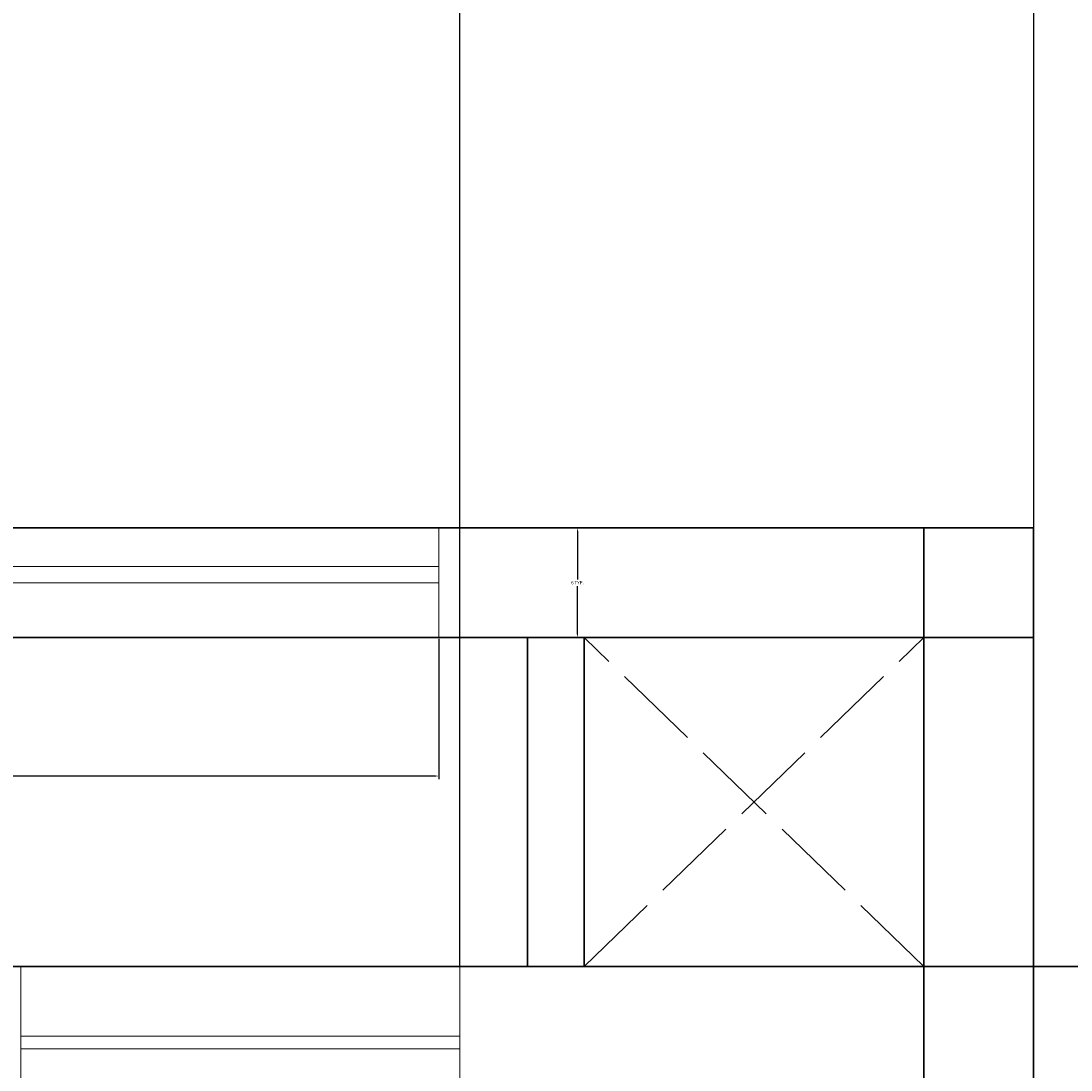
# Model space of a CAD drawing. Units: inches. Extents: x -61 to 1599, y -1316 to 257.
# Tile 73 of 204: x 348 to 406, y -623 to -565. Entities that reach past the tile are written whole.
import ezdxf

# ---------------------------------------------------------------- set-up
doc = ezdxf.new("R2010")
doc.units = ezdxf.units.IN
doc.header["$MEASUREMENT"] = 0
doc.linetypes.add('ACAD_ISO02W100', pattern=[15, 12, -3])
for name, color, linetype, lineweight in [('A-ANNO-DIMS', 2, 'Continuous', 18), ('A-FLOR-OPEN-HIDN', 8, 'ACAD_ISO02W100', 13), ('WALLS', 4, 'Continuous', 35), ('WINDOWS', 220, 'Continuous', 18)]:
    doc.layers.add(name, color=color, linetype=linetype, lineweight=lineweight)
doc.styles.get("Standard").update_dxf_attribs({"font": 'arial.ttf'})
doc.dimstyles.get("Standard").update_dxf_attribs({"dimtxt": 0.18, "dimasz": 0.18, "dimexe": 0.18, "dimexo": 0.0625, "dimgap": 0.09, "dimtad": 0, "dimtih": 1, "dimtoh": 1, "dimdec": 0, "dimzin": 0, "dimdsep": 46, "dimlunit": 3, "dimtxsty": 'Standard', "dimcen": 0.09, "dimadec": 0, "dimazin": 0, "dimtfac": 1, "dimtdec": 0, "dimtofl": 0, "dimtmove": 0, "dimatfit": 3, "dimfxl": 1, "dimtolj": 1, "dimtzin": 0, "dimarcsym": 0})

# ---------------------------------------------------------------- blocks, each defined once
blk = doc.blocks.new('WIN-24IN')
for p, q in [((0, 4.5), (0, 9)), ((0, 9), (0, 0)), ((24, 9), (24, 0)), ((0, 5.192), (24, 5.192)), ((0, 4.5), (24, 4.5))]:
    blk.add_line(p, q)
blk = doc.blocks.new('WIN-51IN')
for p, q in [((0, 0), (0, 6)), ((50.516, 0), (50.516, 6)), ((0, 3.885), (50.516, 3.885)), ((0, 3), (50.516, 3))]:
    blk.add_line(p, q)
blk = doc.blocks.new('*D642')
at = {"layer": 'A-ANNO-DIMS', "color": 0, "lineweight": -2, "transparency": 16777216}
for p, q in [((320.659, -599.007), (320.659, -606.702)), ((371.175, -599.007), (371.175, -606.702)), ((320.839, -606.522), (344.798, -606.522)), ((370.995, -606.522), (347.035, -606.522))]:
    blk.add_line(p, q, dxfattribs=at)
at = {"layer": 'A-ANNO-DIMS', "color": 0, "transparency": 16777216}
for points in [[(320.839, -606.492), (320.839, -606.552), (320.659, -606.522)], [(370.995, -606.492), (370.995, -606.552), (371.175, -606.522)]]:
    blk.add_solid(points, dxfattribs=at)
at = {"layer": 'DEFPOINTS', "color": 0, "transparency": 16777216}
for p in [(320.659, -598.945), (371.175, -598.945), (371.175, -606.522)]:
    blk.add_point(p, dxfattribs=at)
at = {"layer": 'A-ANNO-DIMS', "color": 0, "transparency": 16777216, "insert": (345.917, -606.522), "char_height": 0.18, "attachment_point": 5}
blk.add_mtext('\\A1;WINDOW 51 TYP.', dxfattribs=at)
blk = doc.blocks.new('*D643')
at = {"layer": 'A-ANNO-DIMS', "color": 0, "lineweight": -2, "transparency": 16777216}
for p, q in [((371.237, -592.945), (378.932, -592.945)), ((378.752, -593.125), (378.752, -595.763)), ((378.752, -598.765), (378.752, -596.126)), ((371.237, -598.945), (378.932, -598.945))]:
    blk.add_line(p, q, dxfattribs=at)
at = {"layer": 'A-ANNO-DIMS', "color": 0, "transparency": 16777216}
for points in [[(378.722, -593.125), (378.782, -593.125), (378.752, -592.945)], [(378.722, -598.765), (378.782, -598.765), (378.752, -598.945)]]:
    blk.add_solid(points, dxfattribs=at)
at = {"layer": 'DEFPOINTS', "color": 0, "transparency": 16777216}
for p in [(371.175, -592.945), (378.752, -592.945), (371.175, -598.945)]:
    blk.add_point(p, dxfattribs=at)
at = {"layer": 'A-ANNO-DIMS', "color": 0, "transparency": 16777216, "insert": (378.752, -595.945), "char_height": 0.18, "attachment_point": 5}
blk.add_mtext('\\A1;6 TYP.', dxfattribs=at)
blk = doc.blocks.new('*D703')
at = {"layer": 'A-ANNO-DIMS', "color": 0, "lineweight": -2, "transparency": 16777216}
for p, q in [((372.32, -616.882), (372.32, 257.457)), ((455.833, -616.882), (455.833, 257.457)), ((372.5, 257.277), (413.7, 257.277)), ((455.653, 257.277), (414.453, 257.277))]:
    blk.add_line(p, q, dxfattribs=at)
at = {"layer": 'A-ANNO-DIMS', "color": 0, "transparency": 16777216}
for points in [[(372.5, 257.307), (372.5, 257.247), (372.32, 257.277)], [(455.653, 257.307), (455.653, 257.247), (455.833, 257.277)]]:
    blk.add_solid(points, dxfattribs=at)
at = {"layer": 'DEFPOINTS', "color": 0, "transparency": 16777216}
for p in [(455.833, 257.277), (372.32, -616.945), (455.833, -616.945)]:
    blk.add_point(p, dxfattribs=at)
at = {"layer": 'A-ANNO-DIMS', "color": 0, "transparency": 16777216, "insert": (414.076, 257.277), "char_height": 0.18, "attachment_point": 5}
blk.add_mtext('\\A1;83.51', dxfattribs=at)
blk = doc.blocks.new('*D710')
at = {"layer": 'A-ANNO-DIMS', "color": 0, "lineweight": -2, "transparency": 16777216}
for p, q in [((319.703, -465.385), (319.703, -1315.725)), ((403.703, -465.385), (403.703, -1315.725)), ((319.883, -1315.545), (361.484, -1315.545)), ((403.523, -1315.545), (361.921, -1315.545))]:
    blk.add_line(p, q, dxfattribs=at)
at = {"layer": 'A-ANNO-DIMS', "color": 0, "transparency": 16777216}
for points in [[(319.883, -1315.515), (319.883, -1315.575), (319.703, -1315.545)], [(403.523, -1315.515), (403.523, -1315.575), (403.703, -1315.545)]]:
    blk.add_solid(points, dxfattribs=at)
at = {"layer": 'DEFPOINTS', "color": 0, "transparency": 16777216}
for p in [(319.703, -465.323), (403.703, -465.323), (403.703, -1315.545)]:
    blk.add_point(p, dxfattribs=at)
at = {"layer": 'A-ANNO-DIMS', "color": 0, "transparency": 16777216, "insert": (361.703, -1315.545), "char_height": 0.18, "attachment_point": 5}
blk.add_mtext('\\A1;84', dxfattribs=at)

msp = doc.modelspace()

# ---------------------------------------------------------------- linework, layer by layer
at = {"layer": 'A-FLOR-OPEN-HIDN', "ltscale": 0.4}
for p, q in [((379.1186, -616.9446), (397.7028, -598.9446)), ((397.7028, -616.9446), (379.1186, -598.9446))]:
    msp.add_line(p, q, dxfattribs=at)
at = {"layer": 'WALLS'}
for p, q in [((403.7028, -592.9446), (289.4807, -592.9446)), ((397.7028, -616.9446), (397.7028, -592.9446)), ((403.7028, -616.9446), (403.7028, -592.9446)), ((403.7028, -598.9446), (289.4807, -598.9446)), ((376.0257, -616.9446), (376.0257, -598.9446)), ((379.1186, -616.9446), (379.1186, -598.9446)), ((544.7028, -616.9446), (14.7028, -616.9446)), ((397.7028, -616.9446), (397.7028, -733.9446)), ((403.7028, -616.9446), (403.7028, -733.9446))]:
    msp.add_line(p, q, dxfattribs=at)

# ---------------------------------------------------------------- block references
at = {"layer": 'WINDOWS'}
for name, p in [('WIN-51IN', (320.659, -598.9447)), ('WIN-24IN', (348.3196, -625.9447))]:
    msp.add_blockref(name, p, dxfattribs=at)

# ---------------------------------------------------------------- dimensions: what is measured, and where the dimension line sits
at = {"layer": 'A-ANNO-DIMS'}
for base, p1, p2, override, picture, middle in [((455.8327, 257.2771), (372.3201, -616.9446), (455.8327, -616.9446), {"dimdec": 2, "dimlfac": 1, "dimrnd": 0, "dimzin": 0, "dimdsep": 46, "dimlunit": 2}, '*D703', (414.0764, 257.2771)), ((403.7028, -1315.5446), (319.7028, -465.3229), (403.7028, -465.3229), {"dimdec": 0, "dimlfac": 1, "dimrnd": 0, "dimzin": 0, "dimdsep": 46, "dimlunit": 2}, '*D710', (361.7028, -1315.5446))]:
    dim = msp.add_linear_dim(base=base, p1=p1, p2=p2, dimstyle='Standard', override=override, dxfattribs=at)
    dim.commit()
    dim.dimension.update_dxf_attribs({"geometry": picture, "text_midpoint": middle})
dim = msp.add_linear_dim(base=(378.7519, -592.9446), p1=(371.1745, -598.9446), p2=(371.1745, -592.9446), angle=90, text='<> TYP.', dimstyle='Standard', override={"dimdec": 0, "dimlfac": 1, "dimrnd": 0, "dimzin": 0, "dimdsep": 46, "dimlunit": 2}, dxfattribs=at)
dim.commit()
dim.dimension.update_dxf_attribs({"geometry": '*D643', "text_midpoint": (378.7519, -595.9446)})
dim = msp.add_linear_dim(base=(371.1745, -606.5219), p1=(320.659, -598.9446), p2=(371.1745, -598.9446), text='WINDOW <> TYP.', dimstyle='Standard', override={"dimdec": 0, "dimlfac": 1, "dimrnd": 0, "dimzin": 0, "dimdsep": 46, "dimlunit": 2}, dxfattribs=at)
dim.commit()
dim.dimension.update_dxf_attribs({"geometry": '*D642', "text_midpoint": (345.9168, -606.5219)})

doc.saveas('drawing.dxf')
